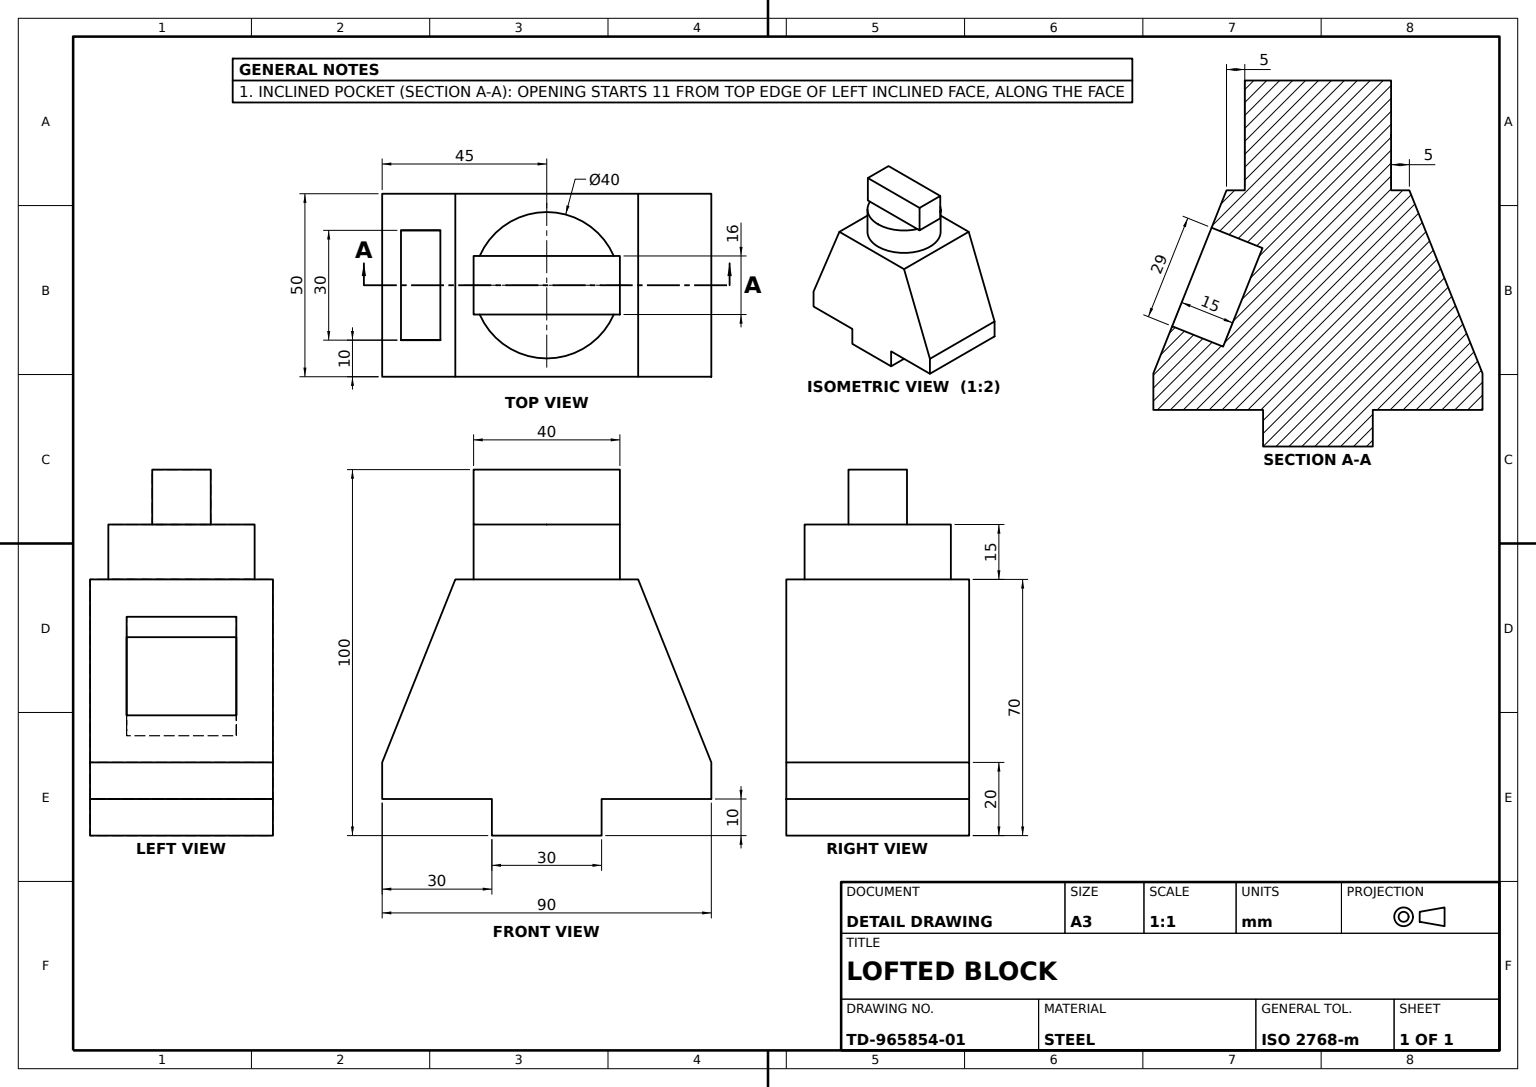
from build123d import *

# Parameters (mm, degrees)
BASE_BLOCK_DEPTH    = 50
ROUND_BOSS_SKETCH_R = 20
ROUND_BOSS_DEPTH    = 15
TOP_KEY_SKETCH_W    = 40
TOP_KEY_SKETCH_H    = 16
TOP_KEY_DEPTH       = 15
SLOT_SKETCH_W       = 30
SLOT_SKETCH_H       = 29
SLOT_CUT_DEPTH      = 15


with BuildPart() as part:
    # Base Profile Sketch → Base Block (new body)
    with BuildSketch(Plane.XY):
        Polygon((15, -5), (45, -5), (45, 5), (-45, 5), (-45, -5), (-15, -5), (-15, -15), (15, -15), align=None)
    extrude(amount=BASE_BLOCK_DEPTH)

    # Loft Top Profile Sketch → section 0 of tapered_body_loft
    with BuildSketch(Plane(origin=(0, 55, 0), x_dir=(1, 0, 0), z_dir=(0, 1, 0)), mode=Mode.PRIVATE) as tapered_body_loft_s0:
        with BuildLine():
            Line((-25, 0), (25, 0))
            Line((25, 0), (25, -50))
            Line((25, -50), (-25, -50))
            Line((-25, -50), (-25, 0))
        make_face()
    # loft up to a face of the part (tapered_body_loft)
    loft([tapered_body_loft_s0.sketch, part.faces().sort_by_distance((0, 5, 25))[0]])

    # Round Boss Sketch → Round Boss (add)
    with BuildSketch(Plane(origin=(0, 55, 0), x_dir=(1, 0, 0), z_dir=(0, 1, 0))):
        with Locations(Location((0, -25, 0), (0, 0, 270))):
            Circle(ROUND_BOSS_SKETCH_R)
    extrude(amount=ROUND_BOSS_DEPTH)

    # Top Key Sketch → Top Key (add)
    with BuildSketch(Plane(origin=(0, 70, 0), x_dir=(1, 0, 0), z_dir=(0, 1, 0))):
        with Locations((0, -25)):
            Rectangle(TOP_KEY_SKETCH_W, TOP_KEY_SKETCH_H)
    extrude(amount=TOP_KEY_DEPTH)

    # Slot Sketch → Slot Cut (cut)
    with BuildSketch(Plane(origin=(-40.517241379, 16.206896552, 0), x_dir=(0, 0, 1), z_dir=(-0.9284766908852594, 0.37139067635410355, 0))):
        with Locations((25, 16.28145109)):
            Rectangle(SLOT_SKETCH_W, SLOT_SKETCH_H)
    extrude(amount=-SLOT_CUT_DEPTH, mode=Mode.SUBTRACT)


solid = part.part
